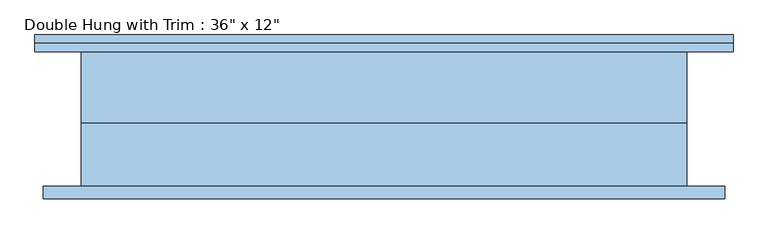
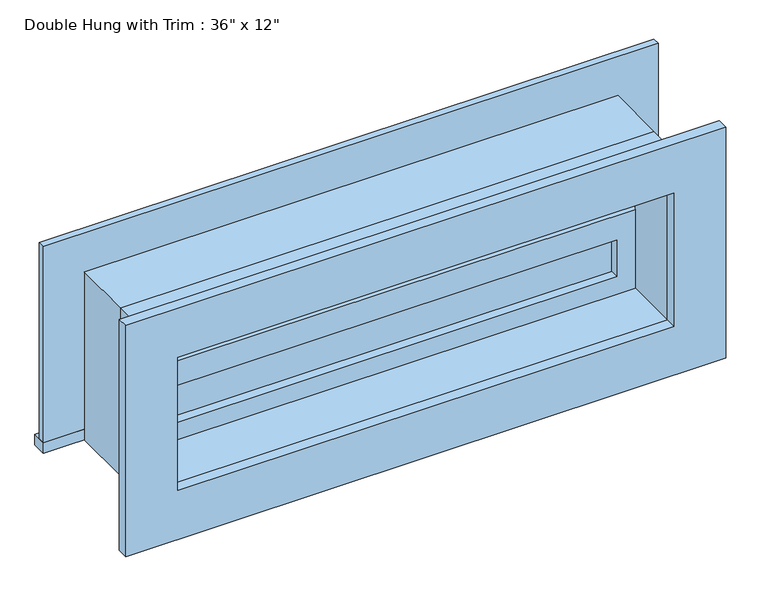
"""IFC4 building model written with IfcOpenShell, lengths in millimetres: window geometry."""

from ifc_helpers import new_model, si_unit, frame, origin, place, context, project, spatial, polyline, outline, extrude, source, transform, mapped, element, save


def window_e4bd14ab(model_context):
    return source(origin(), model_context, "Body", "SweptSolid", [
        extrude(outline(polyline([(-393.7, 22.225), (393.7, 22.225), (393.7, 9.525), (-393.7, 9.525), (-393.7, 22.225)])), frame((0.0, 0.0, 977.9), z_axis=(0.0, 0.0, 1.0), x_axis=(1.0, 0.0, 0.0)), (0.0, 0.0, 1.0), 66.675),
        extrude(outline(polyline([(1089.025, -438.15), (933.45, -438.15), (933.45, 438.15), (1089.025, 438.15), (1089.025, -438.15)]), holes=[polyline([(1044.575, -393.7), (1044.575, 393.7), (977.9, 393.7), (977.9, -393.7), (1044.575, -393.7)])]), frame((0.0, -6.35, 0.0), z_axis=(0.0, 1.0, 0.0), x_axis=(0.0, 0.0, 1.0)), (0.0, 0.0, 1.0), 44.45),
        extrude(outline(polyline([(-527.05, 127.0), (527.05, 127.0), (527.05, 101.6), (-527.05, 101.6), (-527.05, 127.0)])), frame((0.0, 0.0, 914.4), z_axis=(0.0, 0.0, 1.0), x_axis=(1.0, 0.0, 0.0)), (0.0, 0.0, 1.0), 19.05),
        extrude(outline(polyline([(1200.15, -438.15), (1200.15, 438.15), (933.45, 438.15), (933.45, 527.05), (1289.05, 527.05), (1289.05, -527.05), (933.45, -527.05), (933.45, -438.15), (1200.15, -438.15)])), frame((0.0, 101.6, 0.0), z_axis=(0.0, 1.0, 0.0), x_axis=(0.0, 0.0, 1.0)), (0.0, 0.0, 1.0), 12.7),
        extrude(outline(polyline([(1276.35, 514.35), (1276.35, -514.35), (857.25, -514.35), (857.25, 514.35), (1276.35, 514.35)]), holes=[polyline([(1187.45, 425.45), (946.15, 425.45), (946.15, -425.45), (1187.45, -425.45), (1187.45, 425.45)])]), frame((0.0, -120.65, 0.0), z_axis=(0.0, 1.0, 0.0), x_axis=(0.0, 0.0, 1.0)), (0.0, 0.0, 1.0), 19.05),
        extrude(outline(polyline([(393.7, 53.975), (-393.7, 53.975), (-393.7, 66.675), (393.7, 66.675), (393.7, 53.975)])), frame((0.0, 0.0, 1089.025), z_axis=(0.0, 0.0, 1.0), x_axis=(1.0, 0.0, 0.0)), (0.0, 0.0, 1.0), 66.675),
        extrude(outline(polyline([(1200.15, -438.15), (1044.575, -438.15), (1044.575, 438.15), (1200.15, 438.15), (1200.15, -438.15)]), holes=[polyline([(1155.7, -393.7), (1155.7, 393.7), (1089.025, 393.7), (1089.025, -393.7), (1155.7, -393.7)])]), frame((0.0, 38.1, 0.0), z_axis=(0.0, 1.0, 0.0), x_axis=(0.0, 0.0, 1.0)), (0.0, 0.0, 1.0), 44.45),
        extrude(outline(polyline([(1219.2, -457.2), (914.4, -457.2), (914.4, 457.2), (1219.2, 457.2), (1219.2, -457.2)]), holes=[polyline([(1187.45, -425.45), (1187.45, 425.45), (946.15, 425.45), (946.15, -425.45), (1187.45, -425.45)])]), frame((0.0, -101.6, 0.0), z_axis=(0.0, 1.0, 0.0), x_axis=(0.0, 0.0, 1.0)), (0.0, 0.0, 1.0), 95.25),
        extrude(outline(polyline([(1219.2, 457.2), (1219.2, -457.2), (914.4, -457.2), (914.4, 457.2), (1219.2, 457.2)]), holes=[polyline([(1200.15, 438.15), (933.45, 438.15), (933.45, -438.15), (1200.15, -438.15), (1200.15, 438.15)])]), frame((0.0, -6.35, 0.0), z_axis=(0.0, 1.0, 0.0), x_axis=(0.0, 0.0, 1.0)), (0.0, 0.0, 1.0), 107.95),
    ])


if __name__ == "__main__":
    model = new_model("IFC4")
    model_context = context("Model", 3, world=origin())
    ifc_project = project(units=[si_unit("LENGTHUNIT", "METRE", prefix="MILLI")], contexts=[model_context])
    site = spatial("IfcSite", under=ifc_project)
    building = spatial("IfcBuilding", under=site)
    placement = place(None, origin())
    window_shape = window_e4bd14ab(model_context)
    element("IfcWindow", 1, ObjectType="Double Hung with Trim : 36\" x 12\"", at=placement, inside=building, context=model_context, shape_type="MappedRepresentation", body=[
        mapped(window_shape, transform((0.0, 0.0, 0.0), x_axis=(1.0, 0.0, 0.0), y_axis=(0.0, 1.0, 0.0), z_axis=(0.0, 0.0, 1.0))),
    ])
    save(model, "model.ifc")

# Revit data of these elements
# Type "Double Hung with Trim : 36\" x 12\""
#   Type Mark = "21"
#   Construction Type Id = "GSP4R"
#   Assembly Code = "B2020100"
#   Analytic Construction = "1/8 in Pilkington single glazing"
#   Visual Light Transmittance = 0.9
#   Solar Heat Gain Coefficient = 0.78
#   Heat Transfer Coefficient (U) = 0.6496 BTU/(h·ft²·°F)
#   Height = 1' - 0"
#   Default Sill Height = 3' - 0"
#   Trim Projection - Ext. = 0' - 0 1/2"
#   Trim Projection - Int. = 0' - 0 3/4"
#   Trim Width - Exterior = 0' - 3 1/2"
#   Trim Width - Interior = 0' - 3 1/2"
#   Width = 3' - 0"
#   Window Inset = 0' - 0 3/4"
#   Define Thermal Properties by = 1
#   Glass Pane Material = Glass
#   Sash Material = Iron, Ductile
#   Trim Exterior Material = Iron, Ductile
#   Trim Interior Material = Iron, Ductile
#   Wall Closure = (empty or 0)
# Element 1 (IfcWindow, "Double Hung with Trim : 36\" x 12\"")
#   Materials on its faces: "Iron, Ductile", "Glass"
# Materials
#   "Glass": class "Glass", colour RGB 0 128 192, transparency 0.75, Description = "Soda Lime Glass", Cost = 0
#   "Iron, Ductile": class "Metal", colour RGB 0 0 0, transparency 0, Description = "Ductile cast iron", Cost = 0
